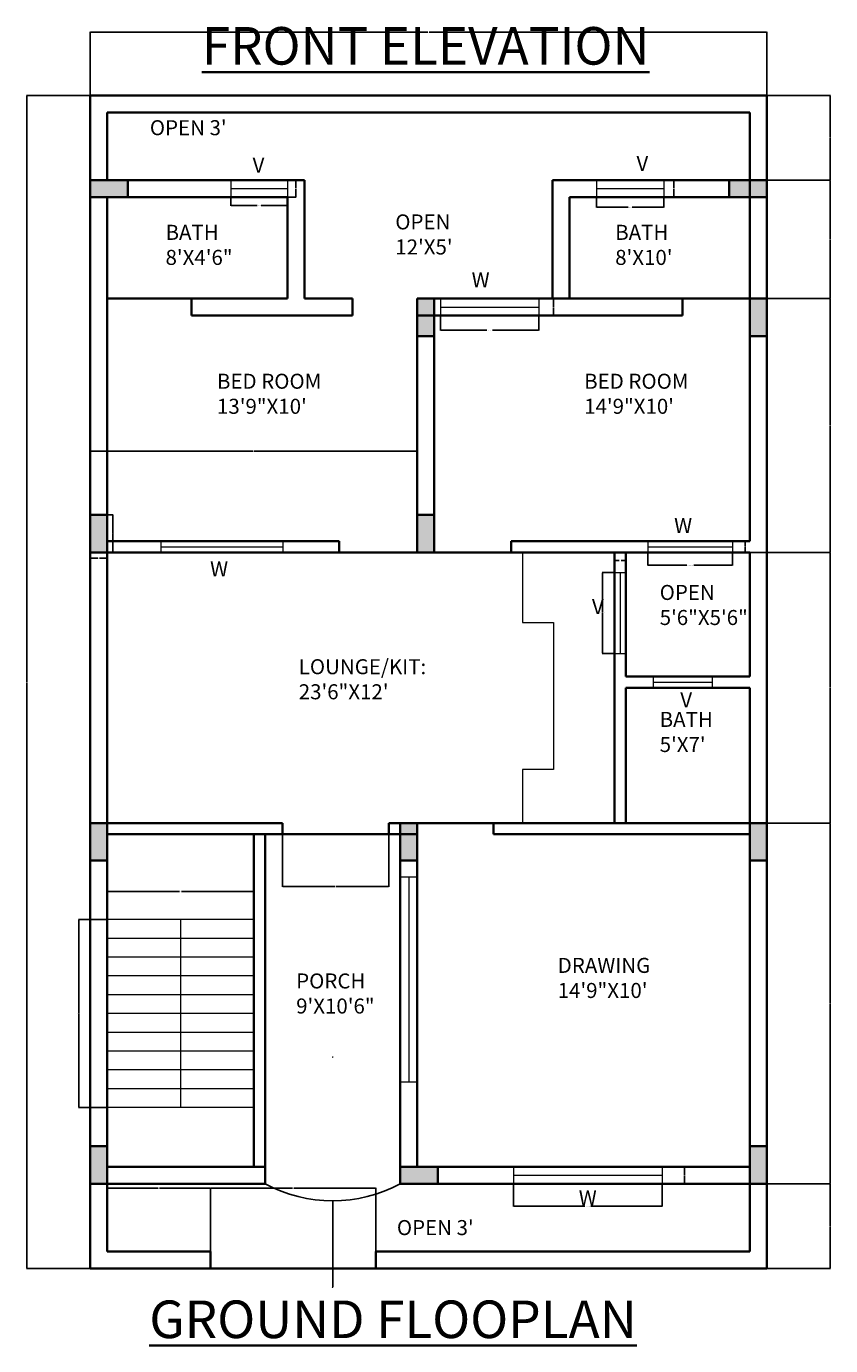
# Model space of a CAD drawing. Units: inches. Extents: x -29 to 834, y -635 to 572.
# Tile 1 of 4: x -29 to 399, y -635 to 66. Entities that reach past the tile are written whole.
import ezdxf

# ---------------------------------------------------------------- set-up
doc = ezdxf.new("R2010")
doc.units = ezdxf.units.IN
doc.header["$MEASUREMENT"] = 0
for name, color, linetype, lineweight in [('A-ANNO-DIMS', 2, 'Continuous', 18), ('A-ANNO-TITL', 7, 'Continuous', 35), ('A-AREA-IDEN', 7, 'Continuous', 18), ('A-COLS', 7, 'Continuous', 35), ('A-FLOR', 7, 'Continuous', 25), ('A-FLOR-FIXT', 8, 'Continuous', 18), ('A-FLOR-STRS', 3, 'Continuous', 18), ('A-GLAZ', 4, 'Continuous', 18), ('A-GLAZ-IDEN', 3, 'Continuous', 18), ('A-WALL', 7, 'Continuous', 35), ('C-PROP', 7, 'Continuous', 35)]:
    doc.layers.add(name, color=color, linetype=linetype, lineweight=lineweight)
doc.styles.get("Standard").update_dxf_attribs({"font": 'arial.ttf'})
doc.dimstyles.get("Standard").update_dxf_attribs({"dimtxt": 0.18, "dimasz": 0.18, "dimexe": 0.18, "dimexo": 0.0625, "dimgap": 0.09, "dimtad": 0, "dimtih": 1, "dimtoh": 1, "dimdec": 4, "dimzin": 0, "dimdsep": 46, "dimtxsty": 'Standard', "dimcen": 0.09, "dimadec": 0, "dimazin": 0, "dimtfac": 1, "dimtdec": 4, "dimtofl": 0, "dimtmove": 0, "dimatfit": 3, "dimfxl": 1, "dimtolj": 1, "dimtzin": 0, "dimarcsym": 0})

# ---------------------------------------------------------------- blocks, each defined once
blk = doc.blocks.new('STAIR-PLAN-RETURN-FLIGHT')
for p, q in [((78, 100), (0, 100)), ((39, 100), (39, 0)), ((78, 90), (0, 90)), ((78, 80), (0, 80)), ((78, 70), (0, 70)), ((78, 60), (0, 60)), ((78, 50), (0, 50)), ((78, 40), (0, 40)), ((78, 30), (0, 30)), ((78, 20), (0, 20)), ((78, 10), (0, 10)), ((78, 0), (0, 0))]:
    blk.add_line(p, q)
blk = doc.blocks.new('KITCHEN-COUNTER-PLAN')
for p, q in [((0, 144), (0, 106.7)), ((0, 106.7), (16.48, 106.7)), ((16.48, 106.7), (16.48, 28.5)), ((16.48, 28.5), (0, 28.5)), ((0, 28.5), (0, 0))]:
    blk.add_line(p, q)
blk = doc.blocks.new('WIN-DRAWING-FRONT-PLAN')
for p, q in [((0, 9), (0, 0)), ((79.05, 9), (79.05, 0)), ((79.05, 4.5), (0, 4.5))]:
    blk.add_line(p, q)
blk = doc.blocks.new('WIN-PORCH-SIDE-PLAN')
for p, q in [((9, 109.08), (0, 109.08)), ((4.5, 0), (4.5, 109.08)), ((9, 0), (0, 0))]:
    blk.add_line(p, q)
blk = doc.blocks.new('WIN-BEDROOM-LOUNGE-PLAN')
for p, q in [((0, 0), (0, 6)), ((64.98, 3), (0, 3)), ((64.98, 0), (64.98, 6))]:
    blk.add_line(p, q)
blk = doc.blocks.new('VENT-LIGHTWELL-SIDE-PLAN')
for p, q in [((6, 43.01), (0, 43.01)), ((3, 0), (3, 43.01)), ((6, 0), (0, 0))]:
    blk.add_line(p, q)
blk = doc.blocks.new('WIN-BEDROOM-REAR-PLAN')
for p, q in [((0, 9), (0, 0)), ((52.22, 9), (52.22, 0)), ((0, 4.5), (52.22, 4.5))]:
    blk.add_line(p, q)
blk = doc.blocks.new('VENT-BATH-LIGHTWELL-PLAN')
for p, q in [((0, 0), (0, 6)), ((31.44, 3), (0, 3)), ((31.44, 0), (31.44, 6))]:
    blk.add_line(p, q)
blk = doc.blocks.new('WIN-BEDROOM-LIGHTWELL-PLAN')
for p, q in [((0, 6), (0, 0)), ((0, 3), (45.04, 3)), ((45.04, 6), (45.04, 0))]:
    blk.add_line(p, q)
blk = doc.blocks.new('VENT-REAR-BATH-R-PLAN')
for p, q in [((0, 9), (0, 0)), ((35.81, 9), (35.81, 0)), ((0, 4.5), (35.81, 4.5))]:
    blk.add_line(p, q)
blk = doc.blocks.new('VENT-REAR-BATH-L-PLAN')
for p, q in [((0, 9), (0, 0)), ((30.05, 9), (30.05, 0)), ((0, 4.5), (30.05, 4.5))]:
    blk.add_line(p, q)
blk = doc.blocks.new('COLUMN-9X20-PLAN')
h = blk.add_hatch(color=256)
h.dxf.hatch_style = 1
h.paths.add_polyline_path([(9, 20), (0, 20), (0, 0), (9, 0)])
blk.add_lwpolyline([(0, 20), (9, 20), (9, 0), (0, 0)], close=True)
blk = doc.blocks.new('*D21')
at = {"layer": 'A-ANNO-DIMS', "color": 0, "lineweight": -2, "transparency": 16777216}
for p, q in [((14.07, -193.46), (17.19, -193.46)), ((17.01, -193.64), (17.01, -203.27)), ((17.01, -213.28), (17.01, -203.64)), ((14.07, -213.46), (17.19, -213.46))]:
    blk.add_line(p, q, dxfattribs=at)
at = {"layer": 'A-ANNO-DIMS', "color": 0, "transparency": 16777216}
for points in [[(16.98, -193.64), (17.04, -193.64), (17.01, -193.46)], [(16.98, -213.28), (17.04, -213.28), (17.01, -213.46)]]:
    blk.add_solid(points, dxfattribs=at)
at = {"layer": 'DEFPOINTS', "color": 0, "transparency": 16777216}
for p in [(14.01, -193.46), (17.01, -193.46), (14.01, -213.46)]:
    blk.add_point(p, dxfattribs=at)
at = {"layer": 'A-ANNO-DIMS', "color": 0, "transparency": 16777216, "insert": (17.01, -203.46), "char_height": 0.18, "attachment_point": 5}
blk.add_mtext('\\A1;COLUMN 20 TYP.', dxfattribs=at)
blk = doc.blocks.new('*D22')
at = {"layer": 'A-ANNO-DIMS', "color": 0, "lineweight": -2, "transparency": 16777216}
for p, q in [((5.01, -213.52), (5.01, -216.64)), ((5.19, -216.46), (9.05, -216.46)), ((13.83, -216.46), (9.97, -216.46)), ((14.01, -213.52), (14.01, -216.64))]:
    blk.add_line(p, q, dxfattribs=at)
at = {"layer": 'A-ANNO-DIMS', "color": 0, "transparency": 16777216}
for points in [[(5.19, -216.43), (5.19, -216.49), (5.01, -216.46)], [(13.83, -216.43), (13.83, -216.49), (14.01, -216.46)]]:
    blk.add_solid(points, dxfattribs=at)
at = {"layer": 'DEFPOINTS', "color": 0, "transparency": 16777216}
for p in [(5.01, -213.46), (14.01, -213.46), (14.01, -216.46)]:
    blk.add_point(p, dxfattribs=at)
at = {"layer": 'A-ANNO-DIMS', "color": 0, "transparency": 16777216, "insert": (9.51, -216.46), "char_height": 0.18, "attachment_point": 5}
blk.add_mtext('\\A1;9 TYP.', dxfattribs=at)
blk = doc.blocks.new('*D23')
at = {"layer": 'A-ANNO-DIMS', "color": 0, "lineweight": -2, "transparency": 16777216}
for p, q in [((13.95, -408.84), (-1.17, -408.84)), ((-0.99, -409.02), (-0.99, -458.66)), ((-0.99, -508.66), (-0.99, -459.03)), ((13.95, -508.84), (-1.17, -508.84))]:
    blk.add_line(p, q, dxfattribs=at)
at = {"layer": 'A-ANNO-DIMS', "color": 0, "transparency": 16777216}
for points in [[(-1.02, -409.02), (-0.96, -409.02), (-0.99, -408.84)], [(-1.02, -508.66), (-0.96, -508.66), (-0.99, -508.84)]]:
    blk.add_solid(points, dxfattribs=at)
at = {"layer": 'DEFPOINTS', "color": 0, "transparency": 16777216}
for p in [(-0.99, -408.84), (14.01, -408.84), (14.01, -508.84)]:
    blk.add_point(p, dxfattribs=at)
at = {"layer": 'A-ANNO-DIMS', "color": 0, "transparency": 16777216, "insert": (-0.99, -458.84), "char_height": 0.18, "attachment_point": 5}
blk.add_mtext('\\A1;FLIGHT 100 TYP.', dxfattribs=at)
blk = doc.blocks.new('*D24')
at = {"layer": 'A-ANNO-DIMS', "color": 0, "lineweight": -2, "transparency": 16777216}
for p, q in [((14.01, -408.78), (14.01, -393.66)), ((14.19, -393.84), (52.48, -393.84)), ((91.83, -393.84), (53.54, -393.84)), ((92.01, -408.78), (92.01, -393.66))]:
    blk.add_line(p, q, dxfattribs=at)
at = {"layer": 'A-ANNO-DIMS', "color": 0, "transparency": 16777216}
for points in [[(14.19, -393.81), (14.19, -393.87), (14.01, -393.84)], [(91.83, -393.81), (91.83, -393.87), (92.01, -393.84)]]:
    blk.add_solid(points, dxfattribs=at)
at = {"layer": 'DEFPOINTS', "color": 0, "transparency": 16777216}
for p in [(92.01, -393.84), (14.01, -408.84), (92.01, -408.84)]:
    blk.add_point(p, dxfattribs=at)
at = {"layer": 'A-ANNO-DIMS', "color": 0, "transparency": 16777216, "insert": (53.01, -393.84), "char_height": 0.18, "attachment_point": 5}
blk.add_mtext('\\A1;78 TYP.', dxfattribs=at)
blk = doc.blocks.new('*D27')
at = {"layer": 'A-ANNO-DIMS', "color": 0, "lineweight": -2, "transparency": 16777216}
for p, q in [((230.26, -549.52), (230.26, -561.49)), ((309.31, -549.52), (309.31, -561.49)), ((230.44, -561.31), (268.21, -561.31)), ((309.13, -561.31), (271.36, -561.31))]:
    blk.add_line(p, q, dxfattribs=at)
at = {"layer": 'A-ANNO-DIMS', "color": 0, "transparency": 16777216}
for points in [[(230.44, -561.28), (230.44, -561.34), (230.26, -561.31)], [(309.13, -561.28), (309.13, -561.34), (309.31, -561.31)]]:
    blk.add_solid(points, dxfattribs=at)
at = {"layer": 'DEFPOINTS', "color": 0, "transparency": 16777216}
for p in [(230.26, -549.46), (309.31, -549.46), (309.31, -561.31)]:
    blk.add_point(p, dxfattribs=at)
at = {"layer": 'A-ANNO-DIMS', "color": 0, "transparency": 16777216, "insert": (269.79, -561.31), "char_height": 0.18, "attachment_point": 5}
blk.add_mtext('\\A1;FRONT WINDOW 79 TYP.', dxfattribs=at)
blk = doc.blocks.new('*D28')
at = {"layer": 'A-ANNO-DIMS', "color": 0, "lineweight": -2, "transparency": 16777216}
for p, q in [((309.37, -540.46), (321.35, -540.46)), ((321.17, -540.64), (321.17, -544.78)), ((321.17, -549.28), (321.17, -545.14)), ((309.37, -549.46), (321.35, -549.46))]:
    blk.add_line(p, q, dxfattribs=at)
at = {"layer": 'A-ANNO-DIMS', "color": 0, "transparency": 16777216}
for points in [[(321.14, -540.64), (321.2, -540.64), (321.17, -540.46)], [(321.14, -549.28), (321.2, -549.28), (321.17, -549.46)]]:
    blk.add_solid(points, dxfattribs=at)
at = {"layer": 'DEFPOINTS', "color": 0, "transparency": 16777216}
for p in [(309.31, -540.46), (321.17, -540.46), (309.31, -549.46)]:
    blk.add_point(p, dxfattribs=at)
at = {"layer": 'A-ANNO-DIMS', "color": 0, "transparency": 16777216, "insert": (321.17, -544.96), "char_height": 0.18, "attachment_point": 5}
blk.add_mtext('\\A1;9 TYP.', dxfattribs=at)
blk = doc.blocks.new('*D33')
at = {"layer": 'A-ANNO-DIMS', "color": 0, "lineweight": -2, "transparency": 16777216}
for p, q in [((283.95, -224.18), (277.38, -224.18)), ((277.56, -224.36), (277.56, -245.51)), ((277.56, -267.02), (277.56, -245.87)), ((283.95, -267.2), (277.38, -267.2))]:
    blk.add_line(p, q, dxfattribs=at)
at = {"layer": 'A-ANNO-DIMS', "color": 0, "transparency": 16777216}
for points in [[(277.53, -224.36), (277.59, -224.36), (277.56, -224.18)], [(277.53, -267.02), (277.59, -267.02), (277.56, -267.2)]]:
    blk.add_solid(points, dxfattribs=at)
at = {"layer": 'DEFPOINTS', "color": 0, "transparency": 16777216}
for p in [(284.01, -224.18), (277.56, -267.2), (284.01, -267.2)]:
    blk.add_point(p, dxfattribs=at)
at = {"layer": 'A-ANNO-DIMS', "color": 0, "transparency": 16777216, "insert": (277.56, -245.69), "char_height": 0.18, "attachment_point": 5}
blk.add_mtext('\\A1;SIDE VENT 43 TYP.', dxfattribs=at)
blk = doc.blocks.new('*D34')
at = {"layer": 'A-ANNO-DIMS', "color": 0, "lineweight": -2, "transparency": 16777216}
for p, q in [((284.01, -224.12), (284.01, -217.55)), ((290.01, -224.12), (290.01, -217.55)), ((284.19, -217.73), (286.55, -217.73)), ((289.83, -217.73), (287.47, -217.73))]:
    blk.add_line(p, q, dxfattribs=at)
at = {"layer": 'A-ANNO-DIMS', "color": 0, "transparency": 16777216}
for points in [[(284.19, -217.7), (284.19, -217.76), (284.01, -217.73)], [(289.83, -217.7), (289.83, -217.76), (290.01, -217.73)]]:
    blk.add_solid(points, dxfattribs=at)
at = {"layer": 'DEFPOINTS', "color": 0, "transparency": 16777216}
for p in [(284.01, -217.73), (284.01, -224.18), (290.01, -224.18)]:
    blk.add_point(p, dxfattribs=at)
at = {"layer": 'A-ANNO-DIMS', "color": 0, "transparency": 16777216, "insert": (287.01, -217.73), "char_height": 0.18, "attachment_point": 5}
blk.add_mtext('\\A1;6 TYP.', dxfattribs=at)
blk = doc.blocks.new('*D35')
at = {"layer": 'A-ANNO-DIMS', "color": 0, "lineweight": -2, "transparency": 16777216}
for p, q in [((191.43, -87.52), (191.43, -95.47)), ((243.65, -87.52), (243.65, -95.47)), ((191.61, -95.29), (216.05, -95.29)), ((243.47, -95.29), (219.04, -95.29))]:
    blk.add_line(p, q, dxfattribs=at)
at = {"layer": 'A-ANNO-DIMS', "color": 0, "transparency": 16777216}
for points in [[(191.61, -95.26), (191.61, -95.32), (191.43, -95.29)], [(243.47, -95.26), (243.47, -95.32), (243.65, -95.29)]]:
    blk.add_solid(points, dxfattribs=at)
at = {"layer": 'DEFPOINTS', "color": 0, "transparency": 16777216}
for p in [(191.43, -87.46), (243.65, -87.46), (243.65, -95.29)]:
    blk.add_point(p, dxfattribs=at)
at = {"layer": 'A-ANNO-DIMS', "color": 0, "transparency": 16777216, "insert": (217.54, -95.29), "char_height": 0.18, "attachment_point": 5}
blk.add_mtext('\\A1;REAR WINDOW 52 TYP.', dxfattribs=at)
blk = doc.blocks.new('*D36')
at = {"layer": 'A-ANNO-DIMS', "color": 0, "lineweight": -2, "transparency": 16777216}
for p, q in [((243.72, -78.46), (251.67, -78.46)), ((251.49, -78.64), (251.49, -82.78)), ((251.49, -87.28), (251.49, -83.14)), ((243.72, -87.46), (251.67, -87.46))]:
    blk.add_line(p, q, dxfattribs=at)
at = {"layer": 'A-ANNO-DIMS', "color": 0, "transparency": 16777216}
for points in [[(251.46, -78.64), (251.52, -78.64), (251.49, -78.46)], [(251.46, -87.28), (251.52, -87.28), (251.49, -87.46)]]:
    blk.add_solid(points, dxfattribs=at)
at = {"layer": 'DEFPOINTS', "color": 0, "transparency": 16777216}
for p in [(243.65, -78.46), (251.49, -78.46), (243.65, -87.46)]:
    blk.add_point(p, dxfattribs=at)
at = {"layer": 'A-ANNO-DIMS', "color": 0, "transparency": 16777216, "insert": (251.49, -82.96), "char_height": 0.18, "attachment_point": 5}
blk.add_mtext('\\A1;9 TYP.', dxfattribs=at)
blk = doc.blocks.new('*D39')
at = {"layer": 'A-ANNO-DIMS', "color": 0, "lineweight": -2, "transparency": 16777216}
for p, q in [((301.76, -213.52), (301.76, -220.39)), ((346.8, -213.52), (346.8, -220.39)), ((301.94, -220.21), (322.42, -220.21)), ((346.62, -220.21), (326.13, -220.21))]:
    blk.add_line(p, q, dxfattribs=at)
at = {"layer": 'A-ANNO-DIMS', "color": 0, "transparency": 16777216}
for points in [[(301.94, -220.18), (301.94, -220.24), (301.76, -220.21)], [(346.62, -220.18), (346.62, -220.24), (346.8, -220.21)]]:
    blk.add_solid(points, dxfattribs=at)
at = {"layer": 'DEFPOINTS', "color": 0, "transparency": 16777216}
for p in [(301.76, -213.46), (346.8, -213.46), (346.8, -220.21)]:
    blk.add_point(p, dxfattribs=at)
at = {"layer": 'A-ANNO-DIMS', "color": 0, "transparency": 16777216, "insert": (324.28, -220.21), "char_height": 0.18, "attachment_point": 5}
blk.add_mtext('\\A1;LIGHTWELL WINDOW 45 TYP.', dxfattribs=at)
blk = doc.blocks.new('*D40')
at = {"layer": 'A-ANNO-DIMS', "color": 0, "lineweight": -2, "transparency": 16777216}
for p, q in [((346.86, -207.46), (353.73, -207.46)), ((353.55, -207.64), (353.55, -210.28)), ((346.86, -213.46), (353.73, -213.46)), ((353.55, -213.28), (353.55, -210.64))]:
    blk.add_line(p, q, dxfattribs=at)
at = {"layer": 'A-ANNO-DIMS', "color": 0, "transparency": 16777216}
for points in [[(353.52, -207.64), (353.58, -207.64), (353.55, -207.46)], [(353.52, -213.28), (353.58, -213.28), (353.55, -213.46)]]:
    blk.add_solid(points, dxfattribs=at)
at = {"layer": 'DEFPOINTS', "color": 0, "transparency": 16777216}
for p in [(346.8, -207.46), (353.55, -207.46), (346.8, -213.46)]:
    blk.add_point(p, dxfattribs=at)
at = {"layer": 'A-ANNO-DIMS', "color": 0, "transparency": 16777216, "insert": (353.55, -210.46), "char_height": 0.18, "attachment_point": 5}
blk.add_mtext('\\A1;6 TYP.', dxfattribs=at)
blk = doc.blocks.new('*D41')
at = {"layer": 'A-ANNO-DIMS', "color": 0, "lineweight": -2, "transparency": 16777216}
for p, q in [((274.45, -24.52), (274.45, -30.01)), ((310.25, -24.52), (310.25, -30.01)), ((274.63, -29.83), (291.24, -29.83)), ((310.07, -29.83), (293.46, -29.83))]:
    blk.add_line(p, q, dxfattribs=at)
at = {"layer": 'A-ANNO-DIMS', "color": 0, "transparency": 16777216}
for points in [[(274.63, -29.8), (274.63, -29.86), (274.45, -29.83)], [(310.07, -29.8), (310.07, -29.86), (310.25, -29.83)]]:
    blk.add_solid(points, dxfattribs=at)
at = {"layer": 'DEFPOINTS', "color": 0, "transparency": 16777216}
for p in [(274.45, -24.46), (310.25, -24.46), (310.25, -29.83)]:
    blk.add_point(p, dxfattribs=at)
at = {"layer": 'A-ANNO-DIMS', "color": 0, "transparency": 16777216, "insert": (292.35, -29.83), "char_height": 0.18, "attachment_point": 5}
blk.add_mtext('\\A1;RH VENT 36 TYP.', dxfattribs=at)
blk = doc.blocks.new('*D42')
at = {"layer": 'A-ANNO-DIMS', "color": 0, "lineweight": -2, "transparency": 16777216}
for p, q in [((310.32, -15.46), (315.81, -15.46)), ((315.63, -15.64), (315.63, -19.78)), ((315.63, -24.28), (315.63, -20.14)), ((310.32, -24.46), (315.81, -24.46))]:
    blk.add_line(p, q, dxfattribs=at)
at = {"layer": 'A-ANNO-DIMS', "color": 0, "transparency": 16777216}
for points in [[(315.6, -15.64), (315.66, -15.64), (315.63, -15.46)], [(315.6, -24.28), (315.66, -24.28), (315.63, -24.46)]]:
    blk.add_solid(points, dxfattribs=at)
at = {"layer": 'DEFPOINTS', "color": 0, "transparency": 16777216}
for p in [(310.25, -15.46), (315.63, -15.46), (310.25, -24.46)]:
    blk.add_point(p, dxfattribs=at)
at = {"layer": 'A-ANNO-DIMS', "color": 0, "transparency": 16777216, "insert": (315.63, -19.96), "char_height": 0.18, "attachment_point": 5}
blk.add_mtext('\\A1;9 TYP.', dxfattribs=at)
blk = doc.blocks.new('*D43')
at = {"layer": 'A-ANNO-DIMS', "color": 0, "lineweight": -2, "transparency": 16777216}
for p, q in [((79.9, -24.52), (79.9, -29.14)), ((109.95, -24.52), (109.95, -29.14)), ((80.08, -28.96), (93.83, -28.96)), ((109.77, -28.96), (96.01, -28.96))]:
    blk.add_line(p, q, dxfattribs=at)
at = {"layer": 'A-ANNO-DIMS', "color": 0, "transparency": 16777216}
for points in [[(80.08, -28.93), (80.08, -28.99), (79.9, -28.96)], [(109.77, -28.93), (109.77, -28.99), (109.95, -28.96)]]:
    blk.add_solid(points, dxfattribs=at)
at = {"layer": 'DEFPOINTS', "color": 0, "transparency": 16777216}
for p in [(79.9, -24.46), (109.95, -24.46), (109.95, -28.96)]:
    blk.add_point(p, dxfattribs=at)
at = {"layer": 'A-ANNO-DIMS', "color": 0, "transparency": 16777216, "insert": (94.92, -28.96), "char_height": 0.18, "attachment_point": 5}
blk.add_mtext('\\A1;LH VENT 30 TYP.', dxfattribs=at)
blk = doc.blocks.new('*D44')
at = {"layer": 'A-ANNO-DIMS', "color": 0, "lineweight": -2, "transparency": 16777216}
for p, q in [((110.01, -15.46), (114.64, -15.46)), ((114.46, -15.64), (114.46, -19.78)), ((114.46, -24.28), (114.46, -20.14)), ((110.01, -24.46), (114.64, -24.46))]:
    blk.add_line(p, q, dxfattribs=at)
at = {"layer": 'A-ANNO-DIMS', "color": 0, "transparency": 16777216}
for points in [[(114.43, -15.64), (114.49, -15.64), (114.46, -15.46)], [(114.43, -24.28), (114.49, -24.28), (114.46, -24.46)]]:
    blk.add_solid(points, dxfattribs=at)
at = {"layer": 'DEFPOINTS', "color": 0, "transparency": 16777216}
for p in [(109.95, -15.46), (114.46, -15.46), (109.95, -24.46)]:
    blk.add_point(p, dxfattribs=at)
at = {"layer": 'A-ANNO-DIMS', "color": 0, "transparency": 16777216, "insert": (114.46, -19.96), "char_height": 0.18, "attachment_point": 5}
blk.add_mtext('\\A1;9 TYP.', dxfattribs=at)
blk = doc.blocks.new('*D59')
at = {"layer": 'A-ANNO-DIMS', "color": 0, "lineweight": -2, "transparency": 16777216}
for p, q in [((5.01, 29.61), (5.01, 63.52)), ((5.19, 63.34), (184.72, 63.34)), ((364.83, 63.34), (185.3, 63.34)), ((365.01, 29.61), (365.01, 63.52))]:
    blk.add_line(p, q, dxfattribs=at)
at = {"layer": 'A-ANNO-DIMS', "color": 0, "transparency": 16777216}
for points in [[(5.19, 63.37), (5.19, 63.31), (5.01, 63.34)], [(364.83, 63.37), (364.83, 63.31), (365.01, 63.34)]]:
    blk.add_solid(points, dxfattribs=at)
at = {"layer": 'DEFPOINTS', "color": 0, "transparency": 16777216}
for p in [(365.01, 63.34), (5.01, 29.54), (365.01, 29.54)]:
    blk.add_point(p, dxfattribs=at)
at = {"layer": 'A-ANNO-DIMS', "color": 0, "transparency": 16777216, "insert": (185.01, 63.34), "char_height": 0.18, "attachment_point": 5}
blk.add_mtext('\\A1;360', dxfattribs=at)
blk = doc.blocks.new('*D60')
at = {"layer": 'A-ANNO-DIMS', "color": 0, "lineweight": -2, "transparency": 16777216}
for p, q in [((4.95, 29.54), (-28.97, 29.54)), ((-28.79, 29.36), (-28.79, -282.28)), ((-28.79, -594.28), (-28.79, -282.64)), ((4.95, -594.46), (-28.97, -594.46))]:
    blk.add_line(p, q, dxfattribs=at)
at = {"layer": 'A-ANNO-DIMS', "color": 0, "transparency": 16777216}
for points in [[(-28.82, 29.36), (-28.76, 29.36), (-28.79, 29.54)], [(-28.82, -594.28), (-28.76, -594.28), (-28.79, -594.46)]]:
    blk.add_solid(points, dxfattribs=at)
at = {"layer": 'DEFPOINTS', "color": 0, "transparency": 16777216}
for p in [(-28.79, 29.54), (5.01, 29.54), (5.01, -594.46)]:
    blk.add_point(p, dxfattribs=at)
at = {"layer": 'A-ANNO-DIMS', "color": 0, "transparency": 16777216, "insert": (-28.79, -282.46), "char_height": 0.18, "attachment_point": 5}
blk.add_mtext('\\A1;624', dxfattribs=at)
blk = doc.blocks.new('*D66')
at = {"layer": 'A-ANNO-DIMS', "color": 0, "lineweight": -2, "transparency": 16777216}
for p, q in [((365.07, -357.46), (398.99, -357.46)), ((398.81, -357.64), (398.81, -453.28)), ((398.81, -549.28), (398.81, -453.64)), ((365.07, -549.46), (398.99, -549.46))]:
    blk.add_line(p, q, dxfattribs=at)
at = {"layer": 'A-ANNO-DIMS', "color": 0, "transparency": 16777216}
for points in [[(398.78, -357.64), (398.84, -357.64), (398.81, -357.46)], [(398.78, -549.28), (398.84, -549.28), (398.81, -549.46)]]:
    blk.add_solid(points, dxfattribs=at)
at = {"layer": 'DEFPOINTS', "color": 0, "transparency": 16777216}
for p in [(365.01, -357.46), (398.81, -357.46), (365.01, -549.46)]:
    blk.add_point(p, dxfattribs=at)
at = {"layer": 'A-ANNO-DIMS', "color": 0, "transparency": 16777216, "insert": (398.81, -453.46), "char_height": 0.18, "attachment_point": 5}
blk.add_mtext('\\A1;192', dxfattribs=at)
blk = doc.blocks.new('*D67')
at = {"layer": 'A-ANNO-DIMS', "color": 0, "lineweight": -2, "transparency": 16777216}
for p, q in [((356.07, -213.46), (398.99, -213.46)), ((398.81, -213.64), (398.81, -285.28)), ((398.81, -357.28), (398.81, -285.64)), ((365.07, -357.46), (398.99, -357.46))]:
    blk.add_line(p, q, dxfattribs=at)
at = {"layer": 'A-ANNO-DIMS', "color": 0, "transparency": 16777216}
for points in [[(398.78, -213.64), (398.84, -213.64), (398.81, -213.46)], [(398.78, -357.28), (398.84, -357.28), (398.81, -357.46)]]:
    blk.add_solid(points, dxfattribs=at)
at = {"layer": 'DEFPOINTS', "color": 0, "transparency": 16777216}
for p in [(356.01, -213.46), (398.81, -213.46), (365.01, -357.46)]:
    blk.add_point(p, dxfattribs=at)
at = {"layer": 'A-ANNO-DIMS', "color": 0, "transparency": 16777216, "insert": (398.81, -285.46), "char_height": 0.18, "attachment_point": 5}
blk.add_mtext('\\A1;144', dxfattribs=at)
blk = doc.blocks.new('*D68')
at = {"layer": 'A-ANNO-DIMS', "color": 0, "lineweight": -2, "transparency": 16777216}
for p, q in [((365.07, -78.46), (398.99, -78.46)), ((398.81, -78.64), (398.81, -145.77)), ((398.81, -213.28), (398.81, -146.14)), ((356.07, -213.46), (398.99, -213.46))]:
    blk.add_line(p, q, dxfattribs=at)
at = {"layer": 'A-ANNO-DIMS', "color": 0, "transparency": 16777216}
for points in [[(398.78, -78.64), (398.84, -78.64), (398.81, -78.46)], [(398.78, -213.28), (398.84, -213.28), (398.81, -213.46)]]:
    blk.add_solid(points, dxfattribs=at)
at = {"layer": 'DEFPOINTS', "color": 0, "transparency": 16777216}
for p in [(365.01, -78.46), (398.81, -78.46), (356.01, -213.46)]:
    blk.add_point(p, dxfattribs=at)
at = {"layer": 'A-ANNO-DIMS', "color": 0, "transparency": 16777216, "insert": (398.81, -145.96), "char_height": 0.18, "attachment_point": 5}
blk.add_mtext('\\A1;135', dxfattribs=at)
blk = doc.blocks.new('*D69')
at = {"layer": 'A-ANNO-DIMS', "color": 0, "lineweight": -2, "transparency": 16777216}
for p, q in [((365.07, -15.46), (398.99, -15.46)), ((398.81, -15.64), (398.81, -46.77)), ((398.81, -78.28), (398.81, -47.14)), ((365.07, -78.46), (398.99, -78.46))]:
    blk.add_line(p, q, dxfattribs=at)
at = {"layer": 'A-ANNO-DIMS', "color": 0, "transparency": 16777216}
for points in [[(398.78, -15.64), (398.84, -15.64), (398.81, -15.46)], [(398.78, -78.28), (398.84, -78.28), (398.81, -78.46)]]:
    blk.add_solid(points, dxfattribs=at)
at = {"layer": 'DEFPOINTS', "color": 0, "transparency": 16777216}
for p in [(365.01, -15.46), (398.81, -15.46), (365.01, -78.46)]:
    blk.add_point(p, dxfattribs=at)
at = {"layer": 'A-ANNO-DIMS', "color": 0, "transparency": 16777216, "insert": (398.81, -46.96), "char_height": 0.18, "attachment_point": 5}
blk.add_mtext('\\A1;63', dxfattribs=at)
blk = doc.blocks.new('*D70')
at = {"layer": 'A-ANNO-DIMS', "color": 0, "lineweight": -2, "transparency": 16777216}
for p, q in [((365.07, -549.46), (398.99, -549.46)), ((398.81, -549.64), (398.81, -571.78)), ((398.81, -594.28), (398.81, -572.14)), ((365.07, -594.46), (398.99, -594.46))]:
    blk.add_line(p, q, dxfattribs=at)
at = {"layer": 'A-ANNO-DIMS', "color": 0, "transparency": 16777216}
for points in [[(398.78, -549.64), (398.84, -549.64), (398.81, -549.46)], [(398.78, -594.28), (398.84, -594.28), (398.81, -594.46)]]:
    blk.add_solid(points, dxfattribs=at)
at = {"layer": 'DEFPOINTS', "color": 0, "transparency": 16777216}
for p in [(365.01, -549.46), (398.81, -549.46), (365.01, -594.46)]:
    blk.add_point(p, dxfattribs=at)
at = {"layer": 'A-ANNO-DIMS', "color": 0, "transparency": 16777216, "insert": (398.81, -571.96), "char_height": 0.18, "attachment_point": 5}
blk.add_mtext('\\A1;45', dxfattribs=at)
blk = doc.blocks.new('*D71')
at = {"layer": 'A-ANNO-DIMS', "color": 0, "lineweight": -2, "transparency": 16777216}
for p, q in [((365.07, 29.54), (398.99, 29.54)), ((398.81, 29.36), (398.81, 7.22)), ((398.81, -15.28), (398.81, 6.86)), ((365.07, -15.46), (398.99, -15.46))]:
    blk.add_line(p, q, dxfattribs=at)
at = {"layer": 'A-ANNO-DIMS', "color": 0, "transparency": 16777216}
for points in [[(398.78, 29.36), (398.84, 29.36), (398.81, 29.54)], [(398.78, -15.28), (398.84, -15.28), (398.81, -15.46)]]:
    blk.add_solid(points, dxfattribs=at)
at = {"layer": 'DEFPOINTS', "color": 0, "transparency": 16777216}
for p in [(365.01, 29.54), (398.81, 29.54), (365.01, -15.46)]:
    blk.add_point(p, dxfattribs=at)
at = {"layer": 'A-ANNO-DIMS', "color": 0, "transparency": 16777216, "insert": (398.81, 7.04), "char_height": 0.18, "attachment_point": 5}
blk.add_mtext('\\A1;45', dxfattribs=at)
blk = doc.blocks.new('*D77')
at = {"layer": 'A-ANNO-DIMS', "color": 0, "lineweight": -2, "transparency": 16777216}
for p, q in [((5.01, -193.39), (5.01, -159.48)), ((5.19, -159.66), (91.73, -159.66)), ((178.83, -159.66), (92.29, -159.66)), ((179.01, -193.39), (179.01, -159.48))]:
    blk.add_line(p, q, dxfattribs=at)
at = {"layer": 'A-ANNO-DIMS', "color": 0, "transparency": 16777216}
for points in [[(5.19, -159.63), (5.19, -159.69), (5.01, -159.66)], [(178.83, -159.63), (178.83, -159.69), (179.01, -159.66)]]:
    blk.add_solid(points, dxfattribs=at)
at = {"layer": 'DEFPOINTS', "color": 0, "transparency": 16777216}
for p in [(179.01, -159.66), (5.01, -193.46), (179.01, -193.46)]:
    blk.add_point(p, dxfattribs=at)
at = {"layer": 'A-ANNO-DIMS', "color": 0, "transparency": 16777216, "insert": (92.01, -159.66), "char_height": 0.18, "attachment_point": 5}
blk.add_mtext('\\A1;174', dxfattribs=at)
blk = doc.blocks.new('*D78')
at = {"layer": 'A-ANNO-DIMS', "color": 0, "lineweight": -2, "transparency": 16777216}
for p, q in [((107.33, -357.52), (107.33, -391.44)), ((163.93, -357.52), (163.93, -391.44)), ((107.51, -391.26), (135.3, -391.26)), ((163.75, -391.26), (135.95, -391.26))]:
    blk.add_line(p, q, dxfattribs=at)
at = {"layer": 'A-ANNO-DIMS', "color": 0, "transparency": 16777216}
for points in [[(107.51, -391.23), (107.51, -391.29), (107.33, -391.26)], [(163.75, -391.23), (163.75, -391.29), (163.93, -391.26)]]:
    blk.add_solid(points, dxfattribs=at)
at = {"layer": 'DEFPOINTS', "color": 0, "transparency": 16777216}
for p in [(107.33, -357.46), (163.93, -357.46), (107.33, -391.26)]:
    blk.add_point(p, dxfattribs=at)
at = {"layer": 'A-ANNO-DIMS', "color": 0, "transparency": 16777216, "insert": (135.63, -391.26), "char_height": 0.18, "attachment_point": 5}
blk.add_mtext('\\A1;56.6', dxfattribs=at)
blk = doc.blocks.new('*D80')
at = {"layer": 'A-ANNO-DIMS', "color": 0, "lineweight": -2, "transparency": 16777216}
for p, q in [((69.03, -585.39), (69.03, -551.48)), ((69.21, -551.66), (112.6, -551.66)), ((156.78, -551.66), (113.39, -551.66)), ((156.96, -585.39), (156.96, -551.48))]:
    blk.add_line(p, q, dxfattribs=at)
at = {"layer": 'A-ANNO-DIMS', "color": 0, "transparency": 16777216}
for points in [[(69.21, -551.63), (69.21, -551.69), (69.03, -551.66)], [(156.78, -551.63), (156.78, -551.69), (156.96, -551.66)]]:
    blk.add_solid(points, dxfattribs=at)
at = {"layer": 'DEFPOINTS', "color": 0, "transparency": 16777216}
for p in [(156.96, -551.66), (69.03, -585.46), (156.96, -585.46)]:
    blk.add_point(p, dxfattribs=at)
at = {"layer": 'A-ANNO-DIMS', "color": 0, "transparency": 16777216, "insert": (113, -551.66), "char_height": 0.18, "attachment_point": 5}
blk.add_mtext('\\A1;87.93', dxfattribs=at)
blk = doc.blocks.new('*D81')
at = {"layer": 'A-ANNO-DIMS', "color": 0, "lineweight": -2, "transparency": 16777216}
for p, q in [((14.01, -585.39), (14.01, -551.48)), ((14.19, -551.66), (41.13, -551.66)), ((68.85, -551.66), (41.91, -551.66)), ((69.03, -585.39), (69.03, -551.48))]:
    blk.add_line(p, q, dxfattribs=at)
at = {"layer": 'A-ANNO-DIMS', "color": 0, "transparency": 16777216}
for points in [[(14.19, -551.63), (14.19, -551.69), (14.01, -551.66)], [(68.85, -551.63), (68.85, -551.69), (69.03, -551.66)]]:
    blk.add_solid(points, dxfattribs=at)
at = {"layer": 'DEFPOINTS', "color": 0, "transparency": 16777216}
for p in [(69.03, -551.66), (14.01, -585.46), (69.03, -585.46)]:
    blk.add_point(p, dxfattribs=at)
at = {"layer": 'A-ANNO-DIMS', "color": 0, "transparency": 16777216, "insert": (41.52, -551.66), "char_height": 0.18, "attachment_point": 5}
blk.add_mtext('\\A1;55.02', dxfattribs=at)
blk = doc.blocks.new('*D107')
at = {"layer": 'A-ANNO-DIMS', "color": 0, "lineweight": -2, "transparency": 16777216}
for p, q in [((133.92, -481.96), (134.1, -481.96)), ((134.01, -482.05), (134.01, -481.87)), ((134.01, -604.36), (134.01, -558.64)), ((133.83, -604.36), (134.01, -604.36))]:
    blk.add_line(p, q, dxfattribs=at)
at = {"layer": 'A-ANNO-DIMS', "color": 0, "transparency": 16777216}
blk.add_solid([(133.98, -558.64), (134.04, -558.64), (134.01, -558.46)], dxfattribs=at)
at = {"layer": 'DEFPOINTS', "color": 0, "transparency": 16777216}
for p in [(134.01, -481.96), (134.01, -558.46)]:
    blk.add_point(p, dxfattribs=at)
at = {"layer": 'A-ANNO-DIMS', "color": 0, "transparency": 16777216, "insert": (133.42, -604.36), "char_height": 0.18, "attachment_point": 5}
blk.add_mtext('\\A1;R76.5', dxfattribs=at)

msp = doc.modelspace()

# ---------------------------------------------------------------- linework, layer by layer
at = {"layer": 'A-FLOR'}
msp.add_arc((134.0102, -481.957), 76.5, 241.9275073, 298.0724927, dxfattribs=at)
at = {"layer": 'A-WALL'}
for p, q in [((14.0102, 20.5431), (356.0102, 20.5431)), ((14.0102, 20.5431), (14.0102, -15.4569)), ((356.0102, 20.5431), (356.0102, -78.4569)), ((14.0102, -15.4569), (119.0102, -15.4569)), ((119.0102, -15.4569), (119.0102, -78.4569)), ((251.0102, -15.4569), (251.0102, -78.4569)), ((251.0102, -15.4569), (356.0102, -15.4569)), ((14.0102, -24.4569), (110.0102, -24.4569)), ((14.0102, -24.4569), (14.0102, -78.4569)), ((110.0102, -24.4569), (110.0102, -78.4569)), ((260.0102, -24.4569), (260.0102, -78.4569)), ((260.0102, -24.4569), (356.0102, -24.4569)), ((14.0102, -78.4569), (110.0102, -78.4569)), ((14.0102, -78.4569), (14.0102, -87.4569)), ((58.8524, -78.4569), (58.8524, -87.4569)), ((119.0102, -78.4569), (144.5035, -78.4569)), ((144.5035, -78.4569), (144.5035, -87.4569)), ((179.0102, -78.4569), (179.0102, -207.4569)), ((179.0102, -78.4569), (356.0102, -78.4569)), ((320.1324, -78.4569), (320.1324, -87.4569)), ((356.0102, -78.4569), (356.0102, -87.4569)), ((14.0102, -87.4569), (14.0102, -207.4569)), ((58.8524, -87.4569), (144.5035, -87.4569)), ((179.0102, -87.4569), (320.1324, -87.4569)), ((188.0102, -87.4569), (188.0102, -207.4569)), ((356.0102, -87.4569), (356.0102, -207.4569)), ((14.0102, -207.4569), (137.5541, -207.4569)), ((137.5541, -207.4569), (137.5541, -213.4569)), ((179.0102, -207.4569), (179.0102, -213.4569)), ((188.0102, -207.4569), (188.0102, -213.4569)), ((228.9527, -207.4569), (228.9527, -213.4569)), ((228.9527, -207.4569), (356.0102, -207.4569)), ((14.0102, -213.4569), (356.0102, -213.4569)), ((14.0102, -213.4569), (14.0102, -357.4569)), ((284.0102, -213.4569), (284.0102, -357.4569)), ((290.0102, -213.4569), (290.0102, -279.4569)), ((356.0102, -213.4569), (356.0102, -279.4569)), ((290.0102, -279.4569), (356.0102, -279.4569)), ((290.0102, -285.4569), (356.0102, -285.4569)), ((290.0102, -285.4569), (290.0102, -357.4569)), ((356.0102, -285.4569), (356.0102, -357.4569)), ((14.0102, -357.4569), (107.3272, -357.4569)), ((107.3272, -357.4569), (107.3272, -363.4569)), ((163.927, -357.4569), (163.927, -363.4569)), ((163.927, -357.4569), (356.0102, -357.4569)), ((179.0102, -363.4569), (179.0102, -357.4569)), ((219.6358, -357.4569), (219.6358, -363.4569)), ((14.0102, -363.4569), (179.0102, -363.4569)), ((14.0102, -363.4569), (14.0102, -540.4569)), ((92.0102, -363.4569), (92.0102, -540.4569)), ((98.0102, -363.4569), (98.0102, -549.4569)), ((170.0102, -363.4569), (170.0102, -549.4569)), ((179.0102, -363.4569), (179.0102, -540.4569)), ((219.6358, -363.4569), (356.0102, -363.4569)), ((356.0102, -363.4569), (356.0102, -540.4569)), ((14.0102, -540.4569), (98.0102, -540.4569)), ((170.0102, -540.4569), (356.0102, -540.4569)), ((14.0102, -549.4569), (98.0102, -549.4569)), ((14.0102, -549.4569), (14.0102, -585.4569)), ((170.0102, -549.4569), (356.0102, -549.4569)), ((356.0102, -549.4569), (356.0102, -585.4569)), ((14.0102, -585.4569), (69.031, -585.4569)), ((69.031, -585.4569), (69.031, -594.4569)), ((156.9645, -585.4569), (156.9645, -594.4569)), ((156.9645, -585.4569), (356.0102, -585.4569))]:
    msp.add_line(p, q, dxfattribs=at)
at = {"layer": 'C-PROP'}
for p, q in [((5.0102, 29.5431), (5.0102, -594.4569)), ((5.0102, 29.5431), (365.0102, 29.5431)), ((365.0102, 29.5431), (365.0102, -594.4569)), ((5.0102, -594.4569), (365.0102, -594.4569))]:
    msp.add_line(p, q, dxfattribs=at)

# ---------------------------------------------------------------- block references
at = {"layer": 'A-COLS'}
for p, rotation in [((5.0102, -15.4569), 270.0000000000002), ((345.0102, -15.4569), 270.0000000000002), ((170.0102, -540.4569), 269.9999999999998)]:
    msp.add_blockref('COLUMN-9X20-PLAN', p, dxfattribs=dict(at, rotation=rotation))
for p in [(179.0102, -98.4569), (356.0102, -98.4569), (5.0102, -213.4569), (179.0102, -213.4569), (5.0102, -377.4569), (170.0102, -377.4569), (356.0102, -377.4569), (5.0102, -549.4569), (356.0102, -549.4569)]:
    msp.add_blockref('COLUMN-9X20-PLAN', p, dxfattribs=at)
at = {"layer": 'A-FLOR-FIXT'}
msp.add_blockref('KITCHEN-COUNTER-PLAN', (235.1086, -357.4569), dxfattribs=at)
at = {"layer": 'A-FLOR-STRS'}
msp.add_blockref('STAIR-PLAN-RETURN-FLIGHT', (14.0102, -508.8447), dxfattribs=at)
at = {"layer": 'A-GLAZ'}
for name, p in [('VENT-REAR-BATH-L-PLAN', (79.8976, -24.4569)), ('VENT-REAR-BATH-R-PLAN', (274.4479, -24.4569)), ('WIN-BEDROOM-REAR-PLAN', (191.4313, -87.4569)), ('WIN-BEDROOM-LIGHTWELL-PLAN', (301.7553, -213.4569)), ('WIN-DRAWING-FRONT-PLAN', (230.2626, -549.4569))]:
    msp.add_blockref(name, p, dxfattribs=at)
at = {"layer": 'A-GLAZ', "rotation": 180}
for name, p in [('WIN-BEDROOM-LOUNGE-PLAN', (107.5474, -207.4569)), ('VENT-LIGHTWELL-SIDE-PLAN', (290.0102, -224.1814)), ('VENT-BATH-LIGHTWELL-PLAN', (336.0065, -279.4569)), ('WIN-PORCH-SIDE-PLAN', (179.0102, -386.1664))]:
    msp.add_blockref(name, p, dxfattribs=at)

# ---------------------------------------------------------------- texts
at = {"layer": 'A-ANNO-TITL', "char_height": 20, "attachment_point": 1}
for s, insert in [('{\\LFRONT ELEVATION}', (64.3039, 66.0256)), ('{\\LGROUND FLOOPLAN}', (36.4306, -611.4996))]:
    msp.add_mtext_dynamic_manual_height_columns(s, width=384.972308, gutter_width=1, heights=[0], dxfattribs=dict(at, insert=insert))
at = {"layer": 'A-AREA-IDEN', "char_height": 8, "attachment_point": 1}
for s, insert in [("OPEN 3'", (36.7179, 16.4692)), ("OPEN\\P12'X5'", (167.338, -33.6457)), ('BATH\\P8\'X4\'6"', (45.0684, -39.1901)), ("BATH\\P8'X10'", (284.3708, -39.1901)), ('BED ROOM\\P13\'9"X10\'', (72.4414, -118.4186)), ('BED ROOM\\P14\'9"X10\'', (267.8511, -118.4186)), ('OPEN\\P5\'6"X5\'6"', (308.0364, -230.7819)), ('LOUNGE/KIT:\\P23\'6"X12\'', (115.9564, -270.2979)), ("BATH\\P5'X7'", (308.0364, -298.3415)), ('DRAWING\\P14\'9"X10\'', (253.7711, -429.2086)), ('PORCH\\P9\'X10\'6"', (114.5861, -437.4896)), ("OPEN 3'", (168.1918, -568.7152))]:
    msp.add_mtext_dynamic_manual_height_columns(s, width=92.580232, gutter_width=1, heights=[0], dxfattribs=dict(at, insert=insert))
at = {"layer": 'A-GLAZ-IDEN', "char_height": 8, "attachment_point": 1}
for s, width, insert in [('V', 15.530915, (91.397, -3.4402)), ('V', 15.530915, (295.6769, -2.5018)), ('W', 92.580232, (207.9621, -64.4301)), ('W', 92.580232, (315.7376, -195.1503)), ('W', 92.580232, (68.7694, -218.2872)), ('V', 15.530915, (271.9974, -238.3243)), ('V', 15.530915, (319.0009, -287.9574)), ('W', 92.580232, (264.9751, -552.8615))]:
    msp.add_mtext_dynamic_manual_height_columns(s, width=width, gutter_width=1, heights=[0], dxfattribs=dict(at, insert=insert))

# ---------------------------------------------------------------- dimensions: what is measured, and where the dimension line sits
at = {"layer": 'A-ANNO-DIMS'}
for base, p1, p2, override, picture, middle in [((365.0102, 63.3431), (5.0102, 29.5431), (365.0102, 29.5431), {"dimdec": 0, "dimlfac": 1, "dimrnd": 0, "dimzin": 0, "dimdsep": 46, "dimlunit": 2}, '*D59', (185.0102, 63.3431)), ((179.0102, -159.6569), (5.0102, -193.4569), (179.0102, -193.4569), {"dimdec": 0, "dimlfac": 1, "dimrnd": 0, "dimzin": 0, "dimdsep": 46, "dimlunit": 2}, '*D77', (92.0102, -159.6569)), ((69.031, -551.6569), (14.0102, -585.4569), (69.031, -585.4569), {"dimdec": 2, "dimlfac": 1, "dimrnd": 0, "dimzin": 0, "dimdsep": 46, "dimlunit": 2}, '*D81', (41.5206, -551.6569)), ((156.9645, -551.6569), (69.031, -585.4569), (156.9645, -585.4569), {"dimdec": 2, "dimlfac": 1, "dimrnd": 0, "dimzin": 0, "dimdsep": 46, "dimlunit": 2}, '*D80', (112.9977, -551.6569))]:
    dim = msp.add_linear_dim(base=base, p1=p1, p2=p2, dimstyle='Standard', override=override, dxfattribs=at)
    dim.commit()
    dim.dimension.update_dxf_attribs({"geometry": picture, "text_midpoint": middle})
for base, p1, p2, angle, override, picture, middle in [((-28.7898, 29.5431), (5.0102, -594.4569), (5.0102, 29.5431), 90, {"dimdec": 0, "dimlfac": 1, "dimrnd": 0, "dimzin": 0, "dimdsep": 46, "dimlunit": 2}, '*D60', (-28.7898, -282.4569)), ((398.8102, 29.5431), (365.0102, -15.4569), (365.0102, 29.5431), 90, {"dimdec": 0, "dimlfac": 1, "dimrnd": 0, "dimzin": 0, "dimdsep": 46, "dimlunit": 2}, '*D71', (398.8102, 7.0431)), ((398.8102, -15.4569), (365.0102, -78.4569), (365.0102, -15.4569), 90, {"dimdec": 0, "dimlfac": 1, "dimrnd": 0, "dimzin": 0, "dimdsep": 46, "dimlunit": 2}, '*D69', (398.8102, -46.9569)), ((398.8102, -78.4569), (356.0102, -213.4569), (365.0102, -78.4569), 90, {"dimdec": 0, "dimlfac": 1, "dimrnd": 0, "dimzin": 0, "dimdsep": 46, "dimlunit": 2}, '*D68', (398.8102, -145.9569)), ((398.8102, -213.4569), (365.0102, -357.4569), (356.0102, -213.4569), 90, {"dimdec": 0, "dimlfac": 1, "dimrnd": 0, "dimzin": 0, "dimdsep": 46, "dimlunit": 2}, '*D67', (398.8102, -285.4569)), ((107.3272, -391.2569), (163.927, -357.4569), (107.3272, -357.4569), 180, {"dimdec": 1, "dimlfac": 1, "dimrnd": 0, "dimzin": 0, "dimdsep": 46, "dimlunit": 2}, '*D78', (135.6271, -391.2569)), ((398.8102, -357.4569), (365.0102, -549.4569), (365.0102, -357.4569), 90, {"dimdec": 0, "dimlfac": 1, "dimrnd": 0, "dimzin": 0, "dimdsep": 46, "dimlunit": 2}, '*D66', (398.8102, -453.4569)), ((398.8102, -549.4569), (365.0102, -594.4569), (365.0102, -549.4569), 90, {"dimdec": 0, "dimlfac": 1, "dimrnd": 0, "dimzin": 0, "dimdsep": 46, "dimlunit": 2}, '*D70', (398.8102, -571.9569))]:
    dim = msp.add_linear_dim(base=base, p1=p1, p2=p2, angle=angle, dimstyle='Standard', override=override, dxfattribs=at)
    dim.commit()
    dim.dimension.update_dxf_attribs({"geometry": picture, "text_midpoint": middle})
for base, p1, p2, angle, text, picture, middle in [((114.459, -15.4569), (109.951, -24.4569), (109.951, -15.4569), 90, '<> TYP.', '*D44', (114.459, -19.9569)), ((315.6252, -15.4569), (310.2542, -24.4569), (310.2542, -15.4569), 90, '<> TYP.', '*D42', (315.6252, -19.9569)), ((251.4875, -78.4569), (243.6541, -87.4569), (243.6541, -78.4569), 90, '<> TYP.', '*D36', (251.4875, -82.9569)), ((17.0102, -193.4569), (14.0102, -213.4569), (14.0102, -193.4569), 90, 'COLUMN <> TYP.', '*D21', (17.0102, -203.4569)), ((353.5531, -207.4569), (346.7969, -213.4569), (346.7969, -207.4569), 90, '<> TYP.', '*D40', (353.5531, -210.4569)), ((284.0102, -217.7294), (290.0102, -224.1814), (284.0102, -224.1814), 180, '<> TYP.', '*D34', (287.0102, -217.7294)), ((277.5581, -267.1952), (284.0102, -224.1814), (284.0102, -267.1952), 270, 'SIDE VENT <> TYP.', '*D33', (277.5581, -245.6883)), ((-0.9898, -408.8447), (14.0102, -508.8447), (14.0102, -408.8447), 90, 'FLIGHT <> TYP.', '*D23', (-0.9898, -458.8447)), ((321.165, -540.4569), (309.3082, -549.4569), (309.3082, -540.4569), 90, '<> TYP.', '*D28', (321.165, -544.9569))]:
    dim = msp.add_linear_dim(base=base, p1=p1, p2=p2, angle=angle, text=text, dimstyle='Standard', override={"dimdec": 0, "dimlfac": 1, "dimrnd": 0, "dimzin": 0, "dimdsep": 46, "dimlunit": 2}, dxfattribs=at)
    dim.commit()
    dim.dimension.update_dxf_attribs({"geometry": picture, "text_midpoint": middle})
for base, p1, p2, text, picture, middle in [((109.951, -28.965), (79.8976, -24.4569), (109.951, -24.4569), 'LH VENT <> TYP.', '*D43', (94.9243, -28.965)), ((310.2542, -29.8279), (274.4479, -24.4569), (310.2542, -24.4569), 'RH VENT <> TYP.', '*D41', (292.3511, -29.8279)), ((243.6541, -95.2904), (191.4313, -87.4569), (243.6541, -87.4569), 'REAR WINDOW <> TYP.', '*D35', (217.5427, -95.2904)), ((14.0102, -216.4569), (5.0102, -213.4569), (14.0102, -213.4569), '<> TYP.', '*D22', (9.5102, -216.4569)), ((346.7969, -220.2132), (301.7553, -213.4569), (346.7969, -213.4569), 'LIGHTWELL WINDOW <> TYP.', '*D39', (324.2761, -220.2132)), ((92.0102, -393.8447), (14.0102, -408.8447), (92.0102, -408.8447), '<> TYP.', '*D24', (53.0102, -393.8447)), ((309.3082, -561.3138), (230.2626, -549.4569), (309.3082, -549.4569), 'FRONT WINDOW <> TYP.', '*D27', (269.7854, -561.3138))]:
    dim = msp.add_linear_dim(base=base, p1=p1, p2=p2, text=text, dimstyle='Standard', override={"dimdec": 0, "dimlfac": 1, "dimrnd": 0, "dimzin": 0, "dimdsep": 46, "dimlunit": 2}, dxfattribs=at)
    dim.commit()
    dim.dimension.update_dxf_attribs({"geometry": picture, "text_midpoint": middle})
dim = msp.add_radius_dim(center=(134.0102, -481.957), mpoint=(134.01, -558.4569), dimstyle='Standard', override={"dimdec": 1, "dimlfac": 1, "dimrnd": 0, "dimzin": 0, "dimdsep": 46, "dimlunit": 2}, dxfattribs=at)
dim.commit()
dim.dimension.update_dxf_attribs({"geometry": '*D107', "text_midpoint": (133.4193, -604.3569), "dimtype": 164})

doc.saveas('drawing.dxf')
